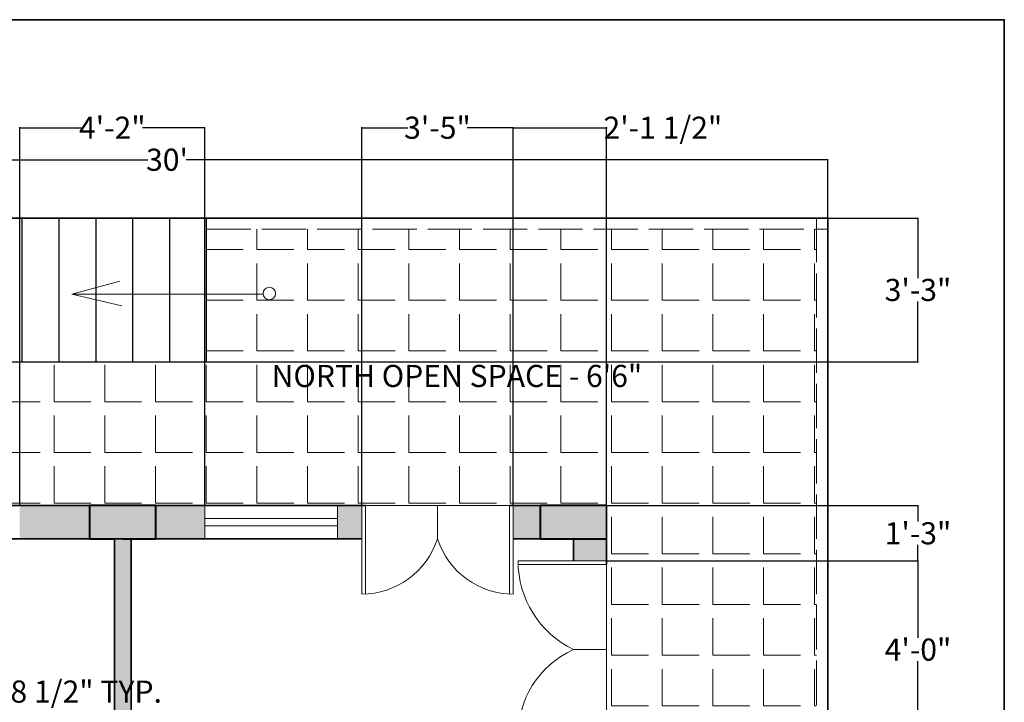
# Model space of a CAD drawing. Units: inches. Extents: x 56944 to 57417, y 173916 to 174454.
# Tile 8 of 8: x 57149 to 57417, y 174268 to 174454. Entities that reach past the tile are written whole.
import ezdxf

# ---------------------------------------------------------------- set-up
doc = ezdxf.new("R2010")
doc.units = ezdxf.units.IN
doc.header["$MEASUREMENT"] = 0
doc.linetypes.add('ACAD_ISO02W100', pattern=[15, 12, -3])
for name, color, linetype, lineweight in [('A-ANNO-DIMS', 2, 'Continuous', 18), ('A-ANNO-SYMB', 7, 'Continuous', 18), ('A-ANNO-TEXT', 7, 'Continuous', 18), ('A-ANNO-TTLB', 7, 'Continuous', 35), ('A-COLS', 7, 'Continuous', 40), ('A-COLS-PATT', 250, 'Continuous', 9), ('A-DOOR', 3, 'Continuous', 20), ('A-FLOR-STRS', 7, 'Continuous', 25), ('A-GLAZ', 4, 'Continuous', 18), ('A-SITE-PATT', 8, 'Continuous', 9), ('A-SITE-WALL-HIDN', 7, 'ACAD_ISO02W100', 18), ('A-WALL', 7, 'Continuous', 35), ('A-WALL-PATT', 241, 'Continuous', 9), ('C-PROP', 7, 'Continuous', 35)]:
    doc.layers.add(name, color=color, linetype=linetype, lineweight=lineweight)
doc.styles.get("Standard").update_dxf_attribs({"font": 'arial.ttf'})
doc.dimstyles.get("Standard").update_dxf_attribs({"dimtxt": 6, "dimasz": 0.18, "dimexe": 0.18, "dimexo": 0.0625, "dimgap": 0.09, "dimtad": 0, "dimtih": 1, "dimtoh": 1, "dimdec": 1, "dimzin": 0, "dimdsep": 46, "dimlunit": 3, "dimtxsty": 'Standard', "dimcen": 0.09, "dimadec": 0, "dimazin": 0, "dimtfac": 1, "dimtdec": 1, "dimtofl": 0, "dimtmove": 0, "dimatfit": 3, "dimfxl": 1, "dimtolj": 1, "dimtzin": 0, "dimarcsym": 0})

# ---------------------------------------------------------------- blocks, each defined once
blk = doc.blocks.new('*D3')
at = {"layer": 'A-ANNO-DIMS', "color": 0, "lineweight": -2, "transparency": 16777216}
for p, q in [((57010.13, 174399.89), (57010.13, 174415.81)), ((57010.31, 174415.63), (57184.2, 174415.63)), ((57368.45, 174415.63), (57194.56, 174415.63)), ((57368.63, 174399.89), (57368.63, 174415.81))]:
    blk.add_line(p, q, dxfattribs=at)
at = {"layer": 'A-ANNO-DIMS', "color": 0, "transparency": 16777216}
for points in [[(57010.31, 174415.66), (57010.31, 174415.6), (57010.13, 174415.63)], [(57368.45, 174415.66), (57368.45, 174415.6), (57368.63, 174415.63)]]:
    blk.add_solid(points, dxfattribs=at)
at = {"layer": 'Defpoints', "color": 0, "transparency": 16777216}
for p in [(57368.63, 174415.63), (57010.13, 174399.82), (57368.63, 174399.82)]:
    blk.add_point(p, dxfattribs=at)
at = {"layer": 'A-ANNO-DIMS', "color": 0, "transparency": 16777216, "insert": (57189.38, 174415.63), "char_height": 6, "attachment_point": 5}
blk.add_mtext("\\A1;30'", dxfattribs=at)
blk = doc.blocks.new('GLAZ-LITE-36IN')
for p, q in [((36, 2), (0, 2)), ((0, 0), (36, 0))]:
    blk.add_line(p, q)
blk = doc.blocks.new('*D16')
at = {"layer": 'A-ANNO-DIMS', "color": 0, "lineweight": -2, "transparency": 16777216}
for p, q in [((57135.34, 174305.75), (57145.76, 174305.75)), ((57145.58, 174305.57), (57145.58, 174274.59)), ((57145.58, 174237.22), (57145.58, 174268.2)), ((57135.34, 174237.04), (57145.76, 174237.04))]:
    blk.add_line(p, q, dxfattribs=at)
at = {"layer": 'A-ANNO-DIMS', "color": 0, "transparency": 16777216}
for points in [[(57145.55, 174305.57), (57145.61, 174305.57), (57145.58, 174305.75)], [(57145.55, 174237.22), (57145.61, 174237.22), (57145.58, 174237.04)]]:
    blk.add_solid(points, dxfattribs=at)
at = {"layer": 'Defpoints', "color": 0, "transparency": 16777216}
for p in [(57135.28, 174305.75), (57145.58, 174305.75), (57135.28, 174237.04)]:
    blk.add_point(p, dxfattribs=at)
at = {"layer": 'A-ANNO-DIMS', "color": 0, "transparency": 16777216, "insert": (57145.58, 174271.39), "char_height": 6, "attachment_point": 5}
blk.add_mtext('\\A1;BED SET 5\'-8 1/2" TYP.', dxfattribs=at)
blk = doc.blocks.new('*D39')
at = {"layer": 'A-ANNO-DIMS', "color": 0, "lineweight": -2, "transparency": 16777216}
for p, q in [((57200.2, 174399.82), (57393.31, 174399.82)), ((57393.13, 174399.64), (57393.13, 174383.48)), ((57393.13, 174361), (57393.13, 174377.17)), ((57200.2, 174360.82), (57393.31, 174360.82))]:
    blk.add_line(p, q, dxfattribs=at)
at = {"layer": 'A-ANNO-DIMS', "color": 0, "transparency": 16777216}
for points in [[(57393.1, 174399.64), (57393.16, 174399.64), (57393.13, 174399.82)], [(57393.1, 174361), (57393.16, 174361), (57393.13, 174360.82)]]:
    blk.add_solid(points, dxfattribs=at)
at = {"layer": 'Defpoints', "color": 0, "transparency": 16777216}
for p in [(57200.13, 174399.82), (57393.13, 174399.82), (57200.13, 174360.82)]:
    blk.add_point(p, dxfattribs=at)
at = {"layer": 'A-ANNO-DIMS', "color": 0, "transparency": 16777216, "insert": (57393.13, 174380.32), "char_height": 6, "attachment_point": 5}
blk.add_mtext('\\A1;3\'-3"', dxfattribs=at)
blk = doc.blocks.new('*D45')
at = {"layer": 'A-ANNO-DIMS', "color": 0, "lineweight": -2, "transparency": 16777216}
for p, q in [((57308.7, 174306.82), (57393.31, 174306.82)), ((57393.13, 174306.64), (57393.13, 174285.93)), ((57393.13, 174258.9), (57393.13, 174279.62)), ((57308.7, 174258.72), (57393.31, 174258.72))]:
    blk.add_line(p, q, dxfattribs=at)
at = {"layer": 'A-ANNO-DIMS', "color": 0, "transparency": 16777216}
for points in [[(57393.1, 174306.64), (57393.16, 174306.64), (57393.13, 174306.82)], [(57393.1, 174258.9), (57393.16, 174258.9), (57393.13, 174258.72)]]:
    blk.add_solid(points, dxfattribs=at)
at = {"layer": 'Defpoints', "color": 0, "transparency": 16777216}
for p in [(57308.63, 174306.82), (57393.13, 174306.82), (57308.63, 174258.72)]:
    blk.add_point(p, dxfattribs=at)
at = {"layer": 'A-ANNO-DIMS', "color": 0, "transparency": 16777216, "insert": (57393.13, 174282.77), "char_height": 6, "attachment_point": 5}
blk.add_mtext('\\A1;4\'-0"', dxfattribs=at)
blk = doc.blocks.new('*D46')
at = {"layer": 'A-ANNO-DIMS', "color": 0, "lineweight": -2, "transparency": 16777216}
for p, q in [((57242.2, 174321.89), (57242.2, 174424.5)), ((57242.38, 174424.32), (57254.7, 174424.32)), ((57283.14, 174424.32), (57270.82, 174424.32)), ((57283.32, 174321.89), (57283.32, 174424.5))]:
    blk.add_line(p, q, dxfattribs=at)
at = {"layer": 'A-ANNO-DIMS', "color": 0, "transparency": 16777216}
for points in [[(57242.38, 174424.35), (57242.38, 174424.29), (57242.2, 174424.32)], [(57283.14, 174424.35), (57283.14, 174424.29), (57283.32, 174424.32)]]:
    blk.add_solid(points, dxfattribs=at)
at = {"layer": 'Defpoints', "color": 0, "transparency": 16777216}
for p in [(57283.32, 174424.32), (57242.2, 174321.82), (57283.32, 174321.82)]:
    blk.add_point(p, dxfattribs=at)
at = {"layer": 'A-ANNO-DIMS', "color": 0, "transparency": 16777216, "insert": (57262.76, 174424.32), "char_height": 6, "attachment_point": 5}
blk.add_mtext('\\A1;3\'-5"', dxfattribs=at)
blk = doc.blocks.new('*D54')
at = {"layer": 'A-ANNO-DIMS', "color": 0, "lineweight": -2, "transparency": 16777216}
for p, q in [((57308.7, 174321.82), (57393.31, 174321.82)), ((57393.13, 174321.64), (57393.13, 174317.48)), ((57393.13, 174307), (57393.13, 174311.17)), ((57308.7, 174306.82), (57393.31, 174306.82))]:
    blk.add_line(p, q, dxfattribs=at)
at = {"layer": 'A-ANNO-DIMS', "color": 0, "transparency": 16777216}
for points in [[(57393.1, 174321.64), (57393.16, 174321.64), (57393.13, 174321.82)], [(57393.1, 174307), (57393.16, 174307), (57393.13, 174306.82)]]:
    blk.add_solid(points, dxfattribs=at)
at = {"layer": 'Defpoints', "color": 0, "transparency": 16777216}
for p in [(57308.63, 174321.82), (57393.13, 174321.82), (57308.63, 174306.82)]:
    blk.add_point(p, dxfattribs=at)
at = {"layer": 'A-ANNO-DIMS', "color": 0, "transparency": 16777216, "insert": (57393.13, 174314.32), "char_height": 6, "attachment_point": 5}
blk.add_mtext('\\A1;1\'-3"', dxfattribs=at)
blk = doc.blocks.new('*D56')
at = {"layer": 'A-ANNO-DIMS', "color": 0, "lineweight": -2, "transparency": 16777216}
for p, q in [((57149.42, 174321.89), (57149.42, 174424.5)), ((57149.6, 174424.32), (57166.35, 174424.32)), ((57199.48, 174424.32), (57182.72, 174424.32)), ((57199.66, 174321.89), (57199.66, 174424.5))]:
    blk.add_line(p, q, dxfattribs=at)
at = {"layer": 'A-ANNO-DIMS', "color": 0, "transparency": 16777216}
for points in [[(57149.6, 174424.35), (57149.6, 174424.29), (57149.42, 174424.32)], [(57199.48, 174424.35), (57199.48, 174424.29), (57199.66, 174424.32)]]:
    blk.add_solid(points, dxfattribs=at)
at = {"layer": 'Defpoints', "color": 0, "transparency": 16777216}
for p in [(57199.66, 174424.32), (57149.42, 174321.82), (57199.66, 174321.82)]:
    blk.add_point(p, dxfattribs=at)
at = {"layer": 'A-ANNO-DIMS', "color": 0, "transparency": 16777216, "insert": (57174.54, 174424.32), "char_height": 6, "attachment_point": 5}
blk.add_mtext('\\A1;4\'-2"', dxfattribs=at)
blk = doc.blocks.new('*D57')
at = {"layer": 'A-ANNO-DIMS', "color": 0, "lineweight": -2, "transparency": 16777216}
for p, q in [((57283.32, 174321.89), (57283.32, 174424.5)), ((57283.5, 174424.32), (57308.45, 174424.32)), ((57308.63, 174321.89), (57308.63, 174424.5)), ((57308.63, 174424.32), (57308.81, 174424.32))]:
    blk.add_line(p, q, dxfattribs=at)
at = {"layer": 'A-ANNO-DIMS', "color": 0, "transparency": 16777216}
for points in [[(57283.5, 174424.35), (57283.5, 174424.29), (57283.32, 174424.32)], [(57308.45, 174424.35), (57308.45, 174424.29), (57308.63, 174424.32)]]:
    blk.add_solid(points, dxfattribs=at)
at = {"layer": 'Defpoints', "color": 0, "transparency": 16777216}
for p in [(57308.63, 174424.32), (57283.32, 174321.82), (57308.63, 174321.82)]:
    blk.add_point(p, dxfattribs=at)
at = {"layer": 'A-ANNO-DIMS', "color": 0, "transparency": 16777216, "insert": (57323.92, 174424.32), "char_height": 6, "attachment_point": 5}
blk.add_mtext('\\A1;2\'-1 1/2"', dxfattribs=at)

msp = doc.modelspace()

# ---------------------------------------------------------------- hatches: boundary and pattern name
at = {"layer": 'A-COLS-PATT'}
h = msp.add_hatch(color=256, dxfattribs=at)
h.dxf.hatch_style = 1
h.paths.add_polyline_path([(57052.13, 174321.82), (57034.13, 174321.82), (57034.13, 174312.82), (57052.13, 174312.82)])
h.paths.add_polyline_path([(57186.38, 174321.82), (57168.38, 174321.82), (57168.38, 174312.82), (57175.13, 174312.82), (57186.38, 174312.82)])
h.paths.add_polyline_path([(57308.63, 174321.82), (57290.63, 174321.82), (57290.63, 174312.82), (57308.63, 174312.82)])
h.paths.add_polyline_path([(57179.63, 174204.82), (57170.63, 174204.82), (57170.63, 174186.82), (57179.63, 174186.82)])
h.paths.add_polyline_path([(57043.13, 174204.82), (57034.13, 174204.82), (57034.13, 174186.82), (57043.13, 174186.82)])
h.paths.add_polyline_path([(57308.63, 174206.32), (57299.63, 174206.32), (57299.63, 174188.32), (57308.63, 174188.32)])
h.paths.add_polyline_path([(57308.63, 174107.87), (57299.63, 174107.87), (57299.63, 174093.93), (57308.63, 174093.93)])
h.paths.add_polyline_path([(57308.63, 173978.32), (57299.63, 173978.32), (57299.63, 173960.32), (57308.63, 173960.32)])
h.paths.add_polyline_path([(57179.63, 173969.32), (57161.63, 173969.32), (57161.63, 173960.32), (57179.63, 173960.32)])
h.paths.add_polyline_path([(57043.13, 173978.32), (57034.13, 173978.32), (57034.13, 173960.32), (57043.13, 173960.32)])
h.paths.add_polyline_path([(57043.13, 174099.82), (57034.13, 174099.82), (57034.13, 174081.82), (57043.13, 174081.82)])
h.paths.add_polyline_path([(57179.63, 174099.82), (57170.63, 174099.82), (57170.63, 174081.82), (57179.63, 174081.82)])
at = {"layer": 'A-SITE-PATT'}
h = msp.add_hatch(dxfattribs=at)
h.set_pattern_fill('ANGLE', color=256, scale=50)
h.set_pattern_definition([(0, (0, 0), (0, 13.75), [10, -3.75]), (90, (0, 0), (-13.75, 8e-16), [10, -3.75])])
h.paths.add_polyline_path([(57365.63, 174396.82), (57200.13, 174396.82), (57200.13, 174379.18), (57215.46, 174379.18, -1.049383), (57218.84, 174379.34, -0.952941), (57215.46, 174379.18), (57200.13, 174379.18), (57200.13, 174360.82), (57140.13, 174360.82), (57140.13, 174321.82), (57149.42, 174321.82), (57243.2, 174321.82), (57282.32, 174321.82), (57283.32, 174321.82), (57308.63, 174321.82), (57308.63, 174305.82), (57308.63, 174259.72), (57308.63, 174258.72), (57308.63, 174252.72), (57308.63, 174216.72), (57308.63, 174099.82), (57308.63, 174093.93), (57308.63, 174081.93), (57308.63, 173969.32), (57365.63, 173969.32)])
h.paths.add_polyline_path([(57341.88, 174114.38), (57341.88, 174209.81), (57329.51, 174209.81), (57329.51, 174114.38)], flags=24)
h.paths.add_polyline_path([(57215.63, 174350.61), (57326.6, 174350.61), (57326.6, 174362.97), (57215.63, 174362.97)], flags=24)
at = {"layer": 'A-WALL-PATT'}
h = msp.add_hatch(color=256, dxfattribs=at)
h.dxf.hatch_style = 1
h.paths.add_polyline_path([(57089.42, 174321.82), (57052.13, 174321.82), (57052.13, 174312.82), (57089.42, 174312.82)])
h.paths.add_polyline_path([(57168.38, 174321.82), (57149.42, 174321.82), (57149.42, 174312.82), (57168.38, 174312.82)])
h.paths.add_polyline_path([(57199.66, 174321.82), (57186.38, 174321.82), (57186.38, 174312.82), (57199.66, 174312.82)])
h.paths.add_polyline_path([(57179.63, 174312.82), (57177.38, 174312.82), (57175.13, 174312.82), (57175.13, 174204.82), (57179.63, 174204.82)])
h.paths.add_polyline_path([(57043.13, 174312.82), (57034.13, 174312.82), (57034.13, 174204.82), (57043.13, 174204.82)])
h.paths.add_polyline_path([(57043.13, 174147.82), (57121.13, 174147.82), (57121.13, 174099.82), (57115.13, 174099.82), (57115.13, 174095.32), (57121.13, 174095.32), (57133.63, 174095.32), (57133.63, 174099.82), (57125.63, 174099.82), (57125.63, 174200.32), (57133.63, 174200.32), (57133.63, 174204.82), (57115.13, 174204.82), (57115.13, 174200.32), (57121.13, 174200.32), (57121.13, 174152.32), (57043.13, 174152.32), (57043.13, 174162.82), (57034.13, 174162.82), (57034.13, 174131.11), (57043.13, 174131.11)])
h.paths.add_polyline_path([(57043.13, 174081.82), (57034.13, 174081.82), (57034.13, 173978.32), (57043.13, 173978.32)])
h.paths.add_polyline_path([(57093.93, 173969.32), (57043.13, 173969.32), (57043.13, 173960.32), (57093.93, 173960.32)])
h.paths.add_polyline_path([(57161.63, 173969.32), (57153.93, 173969.32), (57153.93, 173960.32), (57161.63, 173960.32)])
h.paths.add_polyline_path([(57179.63, 174081.82), (57175.13, 174081.82), (57175.13, 173969.32), (57179.63, 173969.32)])
h.paths.add_polyline_path([(57299.63, 173969.32), (57179.63, 173969.32), (57179.63, 173960.32), (57299.63, 173960.32)])
h.paths.add_polyline_path([(57308.63, 174025.05), (57299.63, 174025.05), (57299.63, 173978.32), (57308.63, 173978.32)])
h.paths.add_polyline_path([(57308.63, 174081.93), (57299.63, 174081.93), (57299.63, 174075.82), (57227.63, 174075.82), (57227.63, 174081.82), (57223.13, 174081.82), (57223.13, 174075.82), (57223.13, 174071.32), (57299.63, 174071.32), (57299.63, 174061.05), (57308.63, 174061.05)])
h.paths.add_polyline_path([(57308.63, 174140.51), (57299.63, 174140.51), (57299.63, 174128.32), (57223.13, 174128.32), (57223.13, 174117.82), (57227.63, 174117.82), (57227.63, 174123.82), (57299.63, 174123.82), (57299.63, 174119.87), (57308.63, 174119.87)])
h.paths.add_polyline_path([(57308.63, 174216.72), (57299.63, 174216.72), (57299.63, 174206.32), (57308.63, 174206.32)])
h.paths.add_polyline_path([(57308.63, 174188.32), (57299.63, 174188.32), (57299.63, 174176.51), (57308.63, 174176.51)])
h.paths.add_polyline_path([(57308.63, 174258.72), (57299.63, 174258.72), (57299.63, 174252.72), (57308.63, 174252.72)])
h.paths.add_polyline_path([(57308.63, 174312.82), (57299.63, 174312.82), (57299.63, 174306.82), (57308.63, 174306.82)])
h.paths.add_polyline_path([(57290.63, 174321.82), (57283.32, 174321.82), (57283.32, 174312.82), (57290.63, 174312.82)])
h.paths.add_polyline_path([(57242.2, 174321.82), (57235.66, 174321.82), (57235.66, 174312.82), (57242.2, 174312.82)])
h.paths.add_polyline_path([(57083.13, 174204.82), (57043.13, 174204.82), (57043.13, 174200.32), (57083.13, 174200.32)], flags=17)
h.paths.add_polyline_path([(57083.13, 174099.82), (57043.13, 174099.82), (57043.13, 174095.32), (57083.13, 174095.32)], flags=0)

# ---------------------------------------------------------------- linework, layer by layer
at = {"layer": 'A-ANNO-SYMB'}
for p, q in [((57163.59, 174379.18), (57176.56, 174382.72)), ((57176.56, 174382.72), (57163.59, 174379.18)), ((57200.13, 174379.18), (57163.59, 174379.18)), ((57163.59, 174379.18), (57215.51, 174379.18)), ((57163.59, 174379.18), (57177.13, 174375.97))]:
    msp.add_line(p, q, dxfattribs=at)
msp.add_circle((57217.14, 174379.34), 1.69, dxfattribs=at)
at = {"layer": 'A-ANNO-TTLB'}
msp.add_lwpolyline([(56943.57, 174453.61), (57416.55, 174453.61), (57416.55, 173915.6), (56943.57, 173915.6)], close=True, dxfattribs=at)
at = {"layer": 'A-COLS'}
for p, q in [((57186.38, 174321.82), (57168.38, 174321.82)), ((57168.38, 174321.82), (57168.38, 174312.82)), ((57186.38, 174312.82), (57186.38, 174321.82)), ((57308.63, 174321.82), (57290.63, 174321.82)), ((57290.63, 174321.82), (57290.63, 174312.82)), ((57168.38, 174312.82), (57175.13, 174312.82)), ((57177.38, 174312.82), (57186.38, 174312.82)), ((57290.63, 174312.82), (57308.63, 174312.82))]:
    msp.add_line(p, q, dxfattribs=at)
at = {"layer": 'A-DOOR'}
for p, q in [((57242.2, 174321.82), (57242.2, 174297.82)), ((57242.2, 174321.82), (57243.2, 174321.82)), ((57243.2, 174321.82), (57243.2, 174297.82)), ((57243.2, 174321.82), (57282.32, 174321.82)), ((57262.76, 174321.82), (57262.76, 174312.82)), ((57282.32, 174321.82), (57282.32, 174297.82)), ((57282.32, 174321.82), (57283.32, 174321.82)), ((57283.32, 174321.82), (57283.32, 174297.82)), ((57308.63, 174306.82), (57284.63, 174306.82)), ((57284.63, 174306.82), (57308.63, 174306.82)), ((57308.63, 174305.82), (57308.63, 174306.82)), ((57284.63, 174305.82), (57308.63, 174305.82)), ((57308.63, 174305.82), (57308.63, 174259.72)), ((57308.63, 174282.77), (57299.63, 174282.77))]:
    msp.add_line(p, q, dxfattribs=at)
for centre, radius, start, end in [((57242.2, 174319.41), 21.58, 270, 342.2385), ((57283.32, 174319.41), 21.58, 197.7615, 270), ((57311.41, 174306.82), 26.78, 180, 243.904), ((57310.15, 174259.51), 25.53, 114.3285, 181.7674)]:
    msp.add_arc(centre, radius, start, end, dxfattribs=at)
at = {"layer": 'A-FLOR-STRS'}
for p, q in [((57150.13, 174360.82), (57150.13, 174399.82)), ((57160.13, 174360.82), (57160.13, 174399.82)), ((57170.13, 174360.82), (57170.13, 174399.82)), ((57180.13, 174360.82), (57180.13, 174399.82)), ((57190.13, 174360.82), (57190.13, 174399.82)), ((57200.13, 174360.82), (57200.13, 174399.82)), ((57070.13, 174360.82), (57200.13, 174360.82))]:
    msp.add_line(p, q, dxfattribs=at)
at = {"layer": 'A-GLAZ'}
for p, q in [((57199.66, 174321.82), (57199.66, 174312.82)), ((57235.66, 174321.82), (57199.66, 174321.82)), ((57235.66, 174312.82), (57235.66, 174321.82)), ((57199.66, 174312.82), (57235.66, 174312.82))]:
    msp.add_line(p, q, dxfattribs=at)
at = {"layer": 'A-SITE-WALL-HIDN'}
for p, q in [((57200.13, 174399.82), (57200.13, 174396.82)), ((57368.63, 174399.82), (57365.63, 174399.82)), ((57365.63, 174399.82), (57365.63, 173969.32)), ((57200.13, 174396.82), (57368.63, 174396.82))]:
    msp.add_line(p, q, dxfattribs=at)
at = {"layer": 'A-WALL'}
for p, q in [((57034.13, 174321.82), (57243.2, 174321.82)), ((57282.32, 174321.82), (57308.63, 174321.82)), ((57308.63, 174321.82), (57308.63, 174305.82)), ((57034.13, 174312.82), (57242.2, 174312.82)), ((57175.13, 174312.82), (57175.13, 174204.82)), ((57175.13, 174312.82), (57179.63, 174312.82)), ((57179.63, 174312.82), (57179.63, 174186.82)), ((57283.32, 174312.82), (57308.63, 174312.82)), ((57299.63, 174312.82), (57299.63, 174306.82)), ((57308.63, 174312.82), (57308.63, 174306.82))]:
    msp.add_line(p, q, dxfattribs=at)
at = {"layer": 'C-PROP'}
for p, q in [((57034.13, 174399.82), (57308.63, 174399.82)), ((57308.63, 174399.82), (57368.63, 174399.82)), ((57368.63, 174399.82), (57368.63, 173960.32))]:
    msp.add_line(p, q, dxfattribs=at)

# ---------------------------------------------------------------- block references
at = {"layer": 'A-GLAZ'}
msp.add_blockref('GLAZ-LITE-36IN', (57199.66, 174316.32), dxfattribs=at)

# ---------------------------------------------------------------- texts
at = {"layer": 'A-ANNO-TEXT', "insert": (57217.77, 174359.99), "char_height": 6, "attachment_point": 1}
msp.add_mtext_dynamic_manual_height_columns('NORTH OPEN SPACE - 6\'6"', width=113.9378, gutter_width=1, heights=[0], dxfattribs=at)

# ---------------------------------------------------------------- dimensions: what is measured, and where the dimension line sits
at = {"layer": 'A-ANNO-DIMS'}
for base, p1, p2, picture, middle in [((57308.63, 174424.32), (57283.32, 174321.82), (57308.63, 174321.82), '*D57', (57323.92, 174424.32)), ((57199.66, 174424.32), (57149.42, 174321.82), (57199.66, 174321.82), '*D56', (57174.54, 174424.32)), ((57283.32, 174424.32), (57242.2, 174321.82), (57283.32, 174321.82), '*D46', (57262.76, 174424.32))]:
    dim = msp.add_linear_dim(base=base, p1=p1, p2=p2, dimstyle='Standard', override={"dimdec": 1, "dimlfac": 1, "dimrnd": 0, "dimzin": 1, "dimdsep": 46, "dimlunit": 4, "dimfrac": 2}, dxfattribs=at)
    dim.commit()
    dim.dimension.update_dxf_attribs({"geometry": picture, "text_midpoint": middle})
dim = msp.add_linear_dim(base=(57368.63, 174415.63), p1=(57010.13, 174399.82), p2=(57368.63, 174399.82), text="30'", dimstyle='Standard', override={"dimclrd": 0, "dimclre": 0, "dimclrt": 0}, dxfattribs=at)
dim.commit()
dim.dimension.update_dxf_attribs({"geometry": '*D3', "text_midpoint": (57189.38, 174415.63)})
for base, p1, p2, picture, middle in [((57393.13, 174399.82), (57200.13, 174360.82), (57200.13, 174399.82), '*D39', (57393.13, 174380.32)), ((57393.13, 174321.82), (57308.63, 174306.82), (57308.63, 174321.82), '*D54', (57393.13, 174314.32)), ((57393.13, 174306.82), (57308.63, 174258.72), (57308.63, 174306.82), '*D45', (57393.13, 174282.77))]:
    dim = msp.add_linear_dim(base=base, p1=p1, p2=p2, angle=90, dimstyle='Standard', override={"dimdec": 1, "dimlfac": 1, "dimrnd": 0, "dimzin": 1, "dimdsep": 46, "dimlunit": 4, "dimfrac": 2}, dxfattribs=at)
    dim.commit()
    dim.dimension.update_dxf_attribs({"geometry": picture, "text_midpoint": middle})
dim = msp.add_linear_dim(base=(57145.58, 174305.75), p1=(57135.28, 174237.04), p2=(57135.28, 174305.75), angle=90, text='BED SET <> TYP.', dimstyle='Standard', override={"dimdec": 1, "dimlfac": 1, "dimrnd": 0, "dimzin": 1, "dimdsep": 46, "dimlunit": 4, "dimfrac": 2}, dxfattribs=at)
dim.commit()
dim.dimension.update_dxf_attribs({"geometry": '*D16', "text_midpoint": (57145.58, 174271.39)})

doc.saveas('drawing.dxf')
